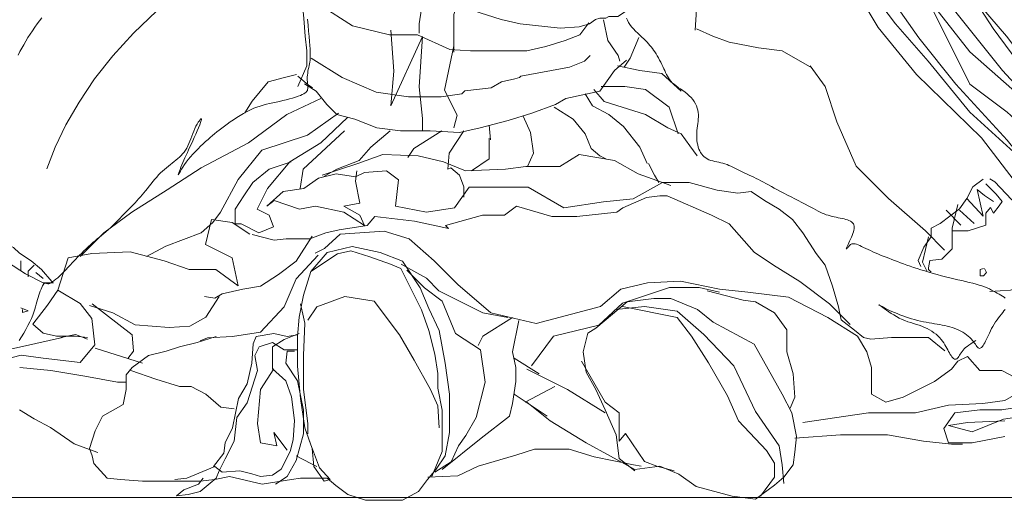
# Model space of a CAD drawing. Units: inches. Extents: x -17 to 1735, y -531 to 60.
# Tile 20 of 27: x 1734.798847 to 1734.807124, y -150.214646 to -150.210609. Entities that reach past the tile are written whole.
import ezdxf

# ---------------------------------------------------------------- set-up
doc = ezdxf.new("R2010")
doc.units = ezdxf.units.IN
doc.header["$MEASUREMENT"] = 0
doc.layers.add('A-FURN', color=242, linetype='Continuous', lineweight=18, true_color=0xcd2027)

# ---------------------------------------------------------------- blocks, each defined once
blk = doc.blocks.new('childrens_room_2')
blk.add_line((73.63163, 54.20212), (73.14631, 54.20212))
for points in [[(73.31539, 54.3045), (73.3149, 54.30385), (73.3144, 54.30318), (73.3139, 54.30247), (73.31339, 54.30174), (73.3129, 54.301), (73.31242, 54.30026), (73.31195, 54.29951), (73.31151, 54.29876), (73.31109, 54.29802), (73.31069, 54.29728), (73.31032, 54.29655)], [(73.31055, 54.23567), (73.31104, 54.23641), (73.31152, 54.23719), (73.31198, 54.238), (73.31242, 54.23882), (73.31281, 54.23962), (73.31315, 54.24037), (73.31344, 54.24107), (73.31368, 54.24171), (73.31387, 54.2423), (73.31404, 54.24286), (73.31418, 54.24338), (73.31431, 54.24388), (73.31444, 54.24436), (73.31457, 54.24483), (73.31471, 54.2453), (73.31487, 54.24576), (73.31503, 54.2462), (73.3152, 54.24661), (73.31537, 54.24698), (73.31553, 54.24729), (73.31569, 54.24754), (73.31583, 54.24772), (73.31596, 54.24782), (73.31609, 54.24785), (73.31621, 54.24785), (73.31634, 54.24781), (73.31649, 54.24777), (73.31666, 54.24775), (73.31686, 54.24776), (73.31709, 54.24782), (73.31737, 54.24796), (73.31768, 54.24816), (73.31802, 54.24841), (73.31839, 54.2487), (73.31876, 54.24902), (73.31914, 54.24937), (73.31951, 54.24972), (73.31988, 54.25008), (73.32022, 54.25043), (73.32056, 54.25078), (73.32088, 54.25112), (73.3212, 54.25147), (73.32153, 54.25182), (73.32187, 54.25219), (73.32223, 54.25257), (73.32261, 54.25297), (73.32302, 54.25339), (73.32345, 54.25384), (73.3239, 54.25429), (73.32437, 54.25475), (73.32485, 54.25521), (73.32533, 54.25567), (73.32581, 54.25611), (73.32629, 54.25654), (73.32676, 54.25694), (73.32722, 54.25732), (73.32768, 54.2577), (73.32813, 54.25807), (73.32859, 54.25845), (73.32906, 54.25884), (73.32953, 54.25925), (73.33002, 54.25969), (73.33052, 54.26015), (73.33103, 54.26065), (73.33154, 54.26116), (73.33206, 54.26169), (73.33256, 54.26221), (73.33306, 54.26273), (73.33355, 54.26324), (73.33401, 54.26373), (73.33445, 54.26419), (73.33488, 54.26462), (73.33528, 54.26504), (73.33567, 54.26545), (73.33605, 54.26586), (73.33642, 54.26627), (73.33679, 54.2667), (73.33717, 54.26714), (73.33754, 54.2676), (73.33792, 54.26808), (73.33831, 54.26858), (73.3387, 54.26907), (73.3391, 54.26957), (73.3395, 54.27005), (73.33991, 54.27052), (73.34032, 54.27097), (73.34074, 54.27139), (73.34115, 54.27178), (73.34157, 54.27215), (73.34199, 54.27251), (73.34241, 54.27284), (73.34282, 54.27317), (73.34323, 54.27349), (73.34363, 54.2738), (73.34402, 54.27412), (73.3444, 54.27444), (73.34476, 54.27477), (73.34511, 54.27511), (73.34544, 54.27547), (73.34575, 54.27585), (73.34604, 54.27625), (73.34631, 54.27669), (73.34655, 54.27716), (73.34678, 54.27766), (73.34699, 54.27817), (73.3472, 54.2787), (73.3474, 54.27924), (73.3476, 54.27978), (73.34782, 54.28032), (73.34804, 54.28084), (73.34829, 54.28134), (73.34854, 54.2818), (73.34878, 54.28221), (73.34901, 54.28254), (73.3492, 54.28279), (73.34935, 54.28293), (73.34944, 54.28295), (73.34946, 54.28283), (73.3494, 54.28256), (73.34927, 54.28215), (73.34908, 54.28164), (73.34884, 54.28104), (73.34856, 54.28038), (73.34826, 54.27968), (73.34794, 54.27897), (73.34762, 54.27827), (73.34731, 54.27759), (73.34701, 54.27695), (73.34672, 54.27634), (73.34645, 54.27575), (73.34618, 54.27519), (73.34593, 54.27464), (73.34569, 54.27411), (73.34547, 54.27359), (73.34526, 54.27309), (73.34507, 54.27261), (73.3449, 54.27216), (73.34476, 54.27177), (73.34465, 54.27144), (73.34457, 54.27119), (73.34452, 54.27103), (73.34452, 54.27097), (73.34457, 54.27103), (73.34465, 54.27119), (73.34479, 54.27145), (73.34497, 54.27178), (73.3452, 54.27219), (73.34548, 54.27265), (73.34582, 54.27316), (73.3462, 54.2737), (73.34664, 54.27426), (73.34713, 54.27483), (73.34764, 54.27541), (73.34818, 54.27598), (73.34873, 54.27655), (73.34929, 54.27709), (73.34983, 54.27762), (73.35036, 54.27811), (73.35086, 54.27856), (73.35133, 54.27899), (73.3518, 54.27939), (73.35227, 54.27977), (73.35275, 54.28016), (73.35325, 54.28054), (73.35378, 54.28094), (73.35435, 54.28136), (73.35496, 54.28181), (73.35562, 54.28227), (73.35631, 54.28275), (73.35702, 54.28322), (73.35774, 54.28368), (73.35847, 54.28411), (73.3592, 54.28452), (73.35992, 54.28488), (73.36062, 54.28519), (73.36131, 54.28545), (73.36198, 54.28567), (73.36265, 54.28587), (73.36332, 54.28604), (73.364, 54.2862), (73.36468, 54.28635), (73.36539, 54.28651), (73.3661, 54.28667), (73.36683, 54.28684), (73.36754, 54.28701), (73.36824, 54.28719), (73.36891, 54.28738), (73.36953, 54.28756), (73.37009, 54.28774), (73.37059, 54.28792), (73.371, 54.2881), (73.37134, 54.28827), (73.3716, 54.28845), (73.37181, 54.28862), (73.37196, 54.28881), (73.37207, 54.28901), (73.37213, 54.28922), (73.37216, 54.28944), (73.37217, 54.28969), (73.37216, 54.28996), (73.37214, 54.29024), (73.37211, 54.29054), (73.37208, 54.29086), (73.37206, 54.29119), (73.37205, 54.29154), (73.37206, 54.29191), (73.37209, 54.29229), (73.37214, 54.29268), (73.37221, 54.29308), (73.37228, 54.29349), (73.37236, 54.29389), (73.37244, 54.29429), (73.37252, 54.29468), (73.37258, 54.29506), (73.37264, 54.29543), (73.37267, 54.29581), (73.37269, 54.29622), (73.3727, 54.29667), (73.37268, 54.29721), (73.37265, 54.29784), (73.3726, 54.29858), (73.37253, 54.29947), (73.37244, 54.30051), (73.37234, 54.30167), (73.37222, 54.30291), (73.37208, 54.30419)], [(73.45448, 54.41111), (73.45858, 54.40576), (73.46299, 54.39757), (73.46709, 54.3897), (73.47119, 54.38214), (73.47718, 54.3708), (73.48475, 54.36198), (73.49042, 54.35222), (73.49894, 54.33301), (73.50907, 54.3176), (73.5138, 54.30941), (73.52137, 54.3006), (73.52894, 54.29052), (73.53745, 54.28044), (73.54596, 54.26974), (73.55353, 54.26029), (73.56456, 54.24769), (73.56734, 54.24595)], [(73.44696, 54.40942), (73.45988, 54.3985), (73.46883, 54.37369), (73.47578, 54.36277), (73.48473, 54.34887), (73.49268, 54.33497), (73.50163, 54.32108), (73.50858, 54.30817), (73.52051, 54.29328), (73.53144, 54.28137), (73.54138, 54.27244), (73.54734, 54.26052), (73.56316, 54.2436)], [(73.42106, 54.40855), (73.42295, 54.40603), (73.42737, 54.39974), (73.43241, 54.39344), (73.44093, 54.38273), (73.44629, 54.37958), (73.45259, 54.37423), (73.45701, 54.36919), (73.46079, 54.36226), (73.46489, 54.35502), (73.46741, 54.34746), (73.46962, 54.34116), (73.47183, 54.33487), (73.47592, 54.32731), (73.48002, 54.32196), (73.48009, 54.32041), (73.48639, 54.31506), (73.49396, 54.30246), (73.50216, 54.29239), (73.51603, 54.27885), (73.52738, 54.26405), (73.54189, 54.24704), (73.54565, 54.24155)], [(73.42509, 54.40843), (73.43702, 54.39652), (73.44994, 54.38163), (73.46088, 54.36376), (73.46783, 54.34887), (73.47479, 54.34291), (73.48175, 54.32505), (73.4887, 54.31512), (73.49765, 54.30321), (73.50461, 54.29527), (73.51355, 54.28435), (73.52448, 54.27442), (73.53343, 54.26549), (73.54138, 54.25358), (73.55157, 54.24155)], [(73.441, 54.40843), (73.44795, 54.40148), (73.45392, 54.38758), (73.46286, 54.37369), (73.46883, 54.35979), (73.47678, 54.34688), (73.48572, 54.33497), (73.49367, 54.32008), (73.5056, 54.30619), (73.51355, 54.2903), (73.5215, 54.28435), (73.53244, 54.27442), (73.53343, 54.27045), (73.54834, 54.25655), (73.55927, 54.24266), (73.5601, 54.24155)], [(73.45094, 54.40843), (73.45789, 54.40049), (73.46584, 54.38858), (73.4738, 54.36277), (73.46982, 54.37766), (73.47877, 54.36475), (73.48572, 54.35086), (73.49268, 54.34192), (73.50063, 54.32703), (73.50958, 54.31611), (73.51852, 54.30222), (73.53244, 54.28336), (73.54436, 54.26946), (73.55629, 54.25556), (73.56679, 54.24595)], [(73.43802, 54.40644), (73.44895, 54.39354), (73.46783, 54.35582), (73.4738, 54.34788), (73.48175, 54.332), (73.4897, 54.32008), (73.49566, 54.31016), (73.50262, 54.30023), (73.51057, 54.2903), (73.5215, 54.27839), (73.52945, 54.26847), (73.53741, 54.26052), (73.54238, 54.25655), (73.54933, 54.24663), (73.55079, 54.24155)], [(73.47578, 54.35185), (73.48672, 54.33696), (73.49765, 54.32306), (73.50262, 54.31115), (73.51355, 54.29725), (73.5225, 54.28931), (73.53343, 54.27541), (73.5384, 54.26847), (73.54436, 54.26449), (73.54834, 54.26052)], [(73.40269, 54.3308), (73.39865, 54.32205), (73.3973, 54.31196), (73.39596, 54.30321), (73.39596, 54.30119), (73.39596, 54.30119)], [(73.40943, 54.32743), (73.40876, 54.32138), (73.40606, 54.3133), (73.40337, 54.30523), (73.40337, 54.30052), (73.40337, 54.29917), (73.40337, 54.29716)], [(73.36676, 54.32146), (73.37149, 54.31862), (73.37591, 54.31673), (73.37938, 54.31642), (73.3819, 54.31516), (73.38568, 54.31296), (73.38915, 54.31233), (73.39419, 54.31044), (73.39829, 54.30981), (73.40302, 54.30729), (73.40744, 54.30603), (73.41343, 54.30414), (73.41753, 54.30319), (73.42604, 54.30225), (73.43014, 54.30256), (73.43235, 54.30319), (73.43361, 54.30414), (73.43455, 54.30445), (73.4355, 54.30445), (73.43581, 54.30445), (73.43644, 54.30477), (73.43834, 54.30477), (73.43999, 54.30587)], [(73.45329, 54.3223), (73.4536, 54.31884), (73.45581, 54.31475), (73.45644, 54.31065), (73.45518, 54.30624), (73.45486, 54.30183)], [(73.3691, 54.31443), (73.37005, 54.31097), (73.37099, 54.30813), (73.37131, 54.30435), (73.37162, 54.30057), (73.37194, 54.29743), (73.37194, 54.29428), (73.37005, 54.28987)], [(73.34543, 54.31061), (73.3399, 54.30598), (73.33493, 54.30121), (73.33052, 54.29635), (73.32665, 54.29144), (73.32332, 54.28652), (73.32051, 54.28166), (73.31823, 54.27689), (73.31646, 54.27226)], [(73.37131, 54.31128), (73.37478, 54.30719), (73.38171, 54.30278), (73.3896, 54.30089), (73.39559, 54.30089), (73.40252, 54.29774), (73.40694, 54.29743), (73.41261, 54.29743), (73.41892, 54.29743), (73.42302, 54.29837), (73.42712, 54.29963), (73.43027, 54.30089), (73.43216, 54.30341)], [(73.44023, 54.30444), (73.44041, 54.30398), (73.44065, 54.30351), (73.44096, 54.30304), (73.44132, 54.30257), (73.44173, 54.30211), (73.44216, 54.30165), (73.44261, 54.30121), (73.44306, 54.30078), (73.44349, 54.30038), (73.44391, 54.29999), (73.44428, 54.29963), (73.44462, 54.29928), (73.44494, 54.29895), (73.44523, 54.29862), (73.4455, 54.29829), (73.44576, 54.29795), (73.44602, 54.29759), (73.44627, 54.29721), (73.44653, 54.2968), (73.44679, 54.29637), (73.44705, 54.29592), (73.4473, 54.29547), (73.44755, 54.295), (73.44779, 54.29454), (73.44801, 54.29408), (73.44822, 54.29364), (73.4484, 54.29322), (73.44858, 54.29281), (73.44876, 54.29242), (73.44895, 54.29205), (73.44916, 54.29168), (73.4494, 54.29133), (73.44968, 54.29099), (73.45, 54.29065), (73.45038, 54.29032), (73.45081, 54.28999), (73.45127, 54.28965), (73.45176, 54.28932), (73.45225, 54.28897), (73.45273, 54.28862), (73.45319, 54.28825), (73.45363, 54.28787), (73.45402, 54.28747), (73.45437, 54.28704), (73.45467, 54.28661), (73.45493, 54.28616), (73.45514, 54.28571), (73.45531, 54.28524), (73.45544, 54.28477), (73.45552, 54.2843), (73.45556, 54.28383), (73.45556, 54.28335), (73.45553, 54.28288), (73.45549, 54.2824), (73.45543, 54.28191), (73.45536, 54.28142), (73.4553, 54.28092), (73.45526, 54.28042), (73.45523, 54.2799), (73.45522, 54.27938), (73.45523, 54.27886), (73.45527, 54.27835), (73.45533, 54.27785), (73.45542, 54.27737), (73.45553, 54.27691), (73.45568, 54.27648), (73.45585, 54.27608), (73.45605, 54.27572), (73.45628, 54.27539), (73.45654, 54.27509), (73.45682, 54.27483), (73.45713, 54.2746), (73.45747, 54.27439), (73.45783, 54.27422), (73.45822, 54.27408), (73.45862, 54.27396), (73.45905, 54.27385), (73.45948, 54.27376), (73.45992, 54.27366), (73.46037, 54.27357), (73.46081, 54.27346), (73.46125, 54.27333), (73.46168, 54.27318), (73.4621, 54.27301), (73.46252, 54.27282), (73.46293, 54.27262), (73.46334, 54.27241), (73.46376, 54.27219), (73.46418, 54.27197), (73.46461, 54.27176), (73.46505, 54.27154), (73.4655, 54.27133), (73.46596, 54.27112), (73.46642, 54.2709), (73.4669, 54.27068), (73.46739, 54.27046), (73.46789, 54.27022), (73.46839, 54.26997), (73.46891, 54.26971), (73.46944, 54.26943), (73.46999, 54.26914), (73.47056, 54.26883), (73.47116, 54.26851), (73.47178, 54.26817), (73.47243, 54.26782), (73.47312, 54.26745), (73.47385, 54.26707), (73.47461, 54.26668), (73.47537, 54.26629), (73.47615, 54.26589), (73.47691, 54.2655), (73.47765, 54.26512), (73.47835, 54.26475), (73.47901, 54.26441), (73.47961, 54.26409), (73.48016, 54.26379), (73.48067, 54.26351), (73.48115, 54.26326), (73.4816, 54.26304), (73.48203, 54.26283), (73.48245, 54.26265), (73.48287, 54.26249), (73.48329, 54.26235), (73.48373, 54.26223), (73.48416, 54.26212), (73.48459, 54.26203), (73.48502, 54.26194), (73.48545, 54.26185), (73.48587, 54.26177), (73.48627, 54.26168), (73.48667, 54.26159), (73.48705, 54.26149), (73.4874, 54.26137), (73.48773, 54.26124), (73.48803, 54.2611), (73.48828, 54.26094), (73.4885, 54.26075), (73.48866, 54.26055), (73.48877, 54.26032), (73.48884, 54.26007), (73.48885, 54.25979), (73.48883, 54.25949), (73.48876, 54.25917), (73.48867, 54.25883), (73.48855, 54.25847), (73.4884, 54.25808), (73.48823, 54.25768), (73.48806, 54.25727), (73.48787, 54.25687), (73.4877, 54.25648), (73.48753, 54.25613), (73.48739, 54.25581), (73.48727, 54.25555), (73.48719, 54.25535), (73.48715, 54.25523), (73.48715, 54.25518), (73.48719, 54.25519), (73.48725, 54.25524), (73.48733, 54.25533), (73.48743, 54.25545), (73.48755, 54.25558), (73.48766, 54.25572), (73.48778, 54.25586), (73.48791, 54.25598), (73.48804, 54.25609), (73.48819, 54.25618), (73.48836, 54.25625), (73.48855, 54.25628), (73.48877, 54.25628), (73.48903, 54.25625), (73.48932, 54.25617), (73.48966, 54.25605), (73.49002, 54.2559), (73.49042, 54.25572), (73.49085, 54.25551), (73.49131, 54.25529), (73.49179, 54.25506), (73.49229, 54.25483), (73.49281, 54.25459), (73.49335, 54.25436), (73.49391, 54.25412), (73.49448, 54.25388), (73.49506, 54.25365), (73.49565, 54.25341), (73.49625, 54.25318), (73.49686, 54.25294), (73.49747, 54.2527), (73.4981, 54.25247), (73.49873, 54.25223), (73.49939, 54.25199), (73.50007, 54.25175), (73.50077, 54.2515), (73.5015, 54.25125), (73.50227, 54.251), (73.50308, 54.25074), (73.50392, 54.25048), (73.50478, 54.25022), (73.50567, 54.24996), (73.50657, 54.24971), (73.50747, 54.24946), (73.50837, 54.24923), (73.50926, 54.249), (73.51014, 54.24879), (73.511, 54.2486), (73.51184, 54.24841), (73.51264, 54.24822), (73.51342, 54.24804), (73.51416, 54.24786), (73.51486, 54.24767), (73.51551, 54.24748), (73.51612, 54.24728), (73.51668, 54.24707), (73.51721, 54.24686), (73.5177, 54.24664), (73.51815, 54.24641), (73.51859, 54.24619), (73.519, 54.24597), (73.5194, 54.24575), (73.51979, 54.24554), (73.52016, 54.24533), (73.52051, 54.24512), (73.52083, 54.24491), (73.52111, 54.2447)], [(73.52107, 54.24229), (73.52082, 54.24197), (73.52055, 54.24162), (73.52027, 54.24126), (73.51997, 54.24086), (73.51966, 54.24046), (73.51935, 54.24003), (73.51904, 54.23959), (73.51874, 54.23913), (73.51846, 54.23866), (73.51819, 54.23819), (73.51794, 54.23771), (73.51771, 54.23723), (73.51749, 54.23677), (73.51729, 54.23632), (73.51709, 54.2359), (73.5169, 54.2355), (73.51672, 54.23515), (73.51655, 54.23484), (73.51638, 54.23457), (73.51621, 54.23435), (73.51605, 54.23418), (73.5159, 54.23405), (73.51575, 54.23398), (73.5156, 54.23396), (73.51546, 54.23399), (73.51533, 54.23408), (73.51519, 54.23421), (73.51505, 54.23439), (73.5149, 54.2346), (73.51473, 54.23484), (73.51455, 54.2351), (73.51434, 54.23538), (73.5141, 54.23567), (73.51382, 54.23597), (73.51352, 54.23627), (73.51318, 54.23656), (73.51282, 54.23685), (73.51244, 54.23713), (73.51203, 54.2374), (73.5116, 54.23765), (73.51115, 54.23788), (73.51069, 54.23808), (73.51022, 54.23826), (73.50973, 54.23843), (73.50923, 54.23857), (73.50872, 54.2387), (73.50819, 54.23882), (73.50765, 54.23893), (73.50711, 54.23903), (73.50655, 54.23913), (73.50598, 54.23922), (73.50541, 54.23932), (73.50482, 54.23942), (73.50422, 54.23953), (73.50362, 54.23964), (73.503, 54.23978), (73.50238, 54.23992), (73.50174, 54.24009), (73.5011, 54.24028), (73.50046, 54.24047), (73.49983, 54.24069), (73.4992, 54.24091), (73.49859, 54.24113), (73.498, 54.24137), (73.49744, 54.2416), (73.4969, 54.24184), (73.4964, 54.24207), (73.49593, 54.24229), (73.49551, 54.2425), (73.49514, 54.24269), (73.49481, 54.24287), (73.49455, 54.24301), (73.49434, 54.24313), (73.49419, 54.24321), (73.49411, 54.24325), (73.49409, 54.24326), (73.49414, 54.24322), (73.49425, 54.24315), (73.49443, 54.24303), (73.49466, 54.24287), (73.49497, 54.24265), (73.49533, 54.24239), (73.49576, 54.2421), (73.49623, 54.24177), (73.49674, 54.24143), (73.49729, 54.24109), (73.49786, 54.24075), (73.49846, 54.24043), (73.49907, 54.24013), (73.49968, 54.23988), (73.50029, 54.23965), (73.50091, 54.23945), (73.50152, 54.23926), (73.50212, 54.23907), (73.50271, 54.23888), (73.50329, 54.23868), (73.50385, 54.23845), (73.50439, 54.2382), (73.50491, 54.23793), (73.5054, 54.23763), (73.50587, 54.23731), (73.50631, 54.23697), (73.50672, 54.23662), (73.50709, 54.23625), (73.50742, 54.23588), (73.50772, 54.23551), (73.50798, 54.23513), (73.50822, 54.23475), (73.50843, 54.23438), (73.50862, 54.23402), (73.5088, 54.23366), (73.50898, 54.23332), (73.50916, 54.233), (73.50934, 54.23269), (73.50952, 54.23241), (73.5097, 54.23217), (73.50989, 54.23196), (73.51007, 54.2318), (73.51024, 54.23168), (73.51041, 54.23163), (73.51058, 54.23163), (73.51073, 54.2317), (73.51088, 54.23184), (73.51102, 54.23202), (73.51117, 54.23224), (73.51132, 54.23248), (73.51149, 54.23275), (73.51167, 54.23303), (73.51186, 54.23331), (73.51208, 54.23358), (73.51233, 54.23385), (73.51261, 54.23412), (73.51294, 54.23439), (73.51331, 54.23467), (73.51374, 54.23496), (73.51422, 54.23528), (73.51478, 54.23562)], [(73.43532, 54.30404), (73.43626, 54.29963), (73.43847, 54.29648), (73.43878, 54.29522)], [(73.38989, 54.30187), (73.39057, 54.29312), (73.38989, 54.28572)], [(73.45518, 54.30215), (73.45865, 54.30057), (73.46212, 54.29932), (73.46842, 54.29806), (73.47347, 54.29743), (73.47978, 54.29382)], [(73.38989, 54.28572), (73.39663, 54.30052), (73.39596, 54.28975), (73.39663, 54.28303), (73.39663, 54.28033)], [(73.44288, 54.30026), (73.44099, 54.29585), (73.43973, 54.29396)], [(73.40337, 54.2985), (73.40135, 54.28908), (73.40404, 54.2837), (73.40337, 54.28101)], [(73.4402, 54.29548), (73.43768, 54.29327), (73.43453, 54.28886), (73.42728, 54.28729), (73.42507, 54.28603), (73.42002, 54.28414), (73.41498, 54.28257), (73.40899, 54.28099), (73.40457, 54.28005), (73.39827, 54.28036), (73.39196, 54.28036), (73.38692, 54.28099), (73.38219, 54.28288), (73.3784, 54.28383), (73.3762, 54.28603), (73.37399, 54.28886), (73.37147, 54.29044)], [(73.37289, 54.29585), (73.37951, 54.29176), (73.38676, 54.28861), (73.3937, 54.28766), (73.40063, 54.28766), (73.40505, 54.28829), (73.40568, 54.28892), (73.41135, 54.28955), (73.41356, 54.29081), (73.4164, 54.29144), (73.41734, 54.29176), (73.41766, 54.29207), (73.42806, 54.29396), (73.43122, 54.29522), (73.43248, 54.29648)], [(73.43831, 54.29422), (73.44304, 54.29327), (73.44777, 54.29264), (73.45187, 54.28886)], [(73.47946, 54.29428), (73.48261, 54.28987), (73.48513, 54.28231), (73.48923, 54.27286), (73.49617, 54.26594), (73.50405, 54.25901), (73.50815, 54.25491)], [(73.36973, 54.29239), (73.36721, 54.29176), (73.36374, 54.29081), (73.36027, 54.28672), (73.3587, 54.2842)], [(73.37005, 54.29207), (73.37226, 54.29018), (73.3732, 54.28955)], [(73.43327, 54.28918), (73.43547, 54.28666), (73.43926, 54.2854), (73.4443, 54.28383), (73.44903, 54.28099), (73.45187, 54.27973), (73.45376, 54.27721), (73.45534, 54.27501)], [(73.43484, 54.28981), (73.43989, 54.28981), (73.4443, 54.28918), (73.44935, 54.2854), (73.45124, 54.27973)], [(73.37494, 54.28729), (73.36768, 54.28383), (73.35949, 54.27784), (73.3494, 54.27249), (73.34215, 54.26777), (73.33458, 54.26304), (73.32859, 54.25863), (73.32354, 54.2536)], [(73.43137, 54.28824), (73.43295, 54.28572), (73.43642, 54.28383), (73.43957, 54.28131), (73.44304, 54.2769), (73.44462, 54.27343)], [(73.42475, 54.2854), (73.42885, 54.28288), (73.43137, 54.27973), (73.43264, 54.27658), (73.43453, 54.27501), (73.43579, 54.27438)], [(73.37872, 54.28414), (73.3721, 54.27942), (73.36232, 54.27627), (73.35728, 54.26997), (73.3535, 54.26304), (73.35192, 54.26084), (73.3494, 54.25863), (73.34183, 54.2558), (73.33773, 54.2536)], [(73.38061, 54.2832), (73.37494, 54.27784), (73.36832, 54.27375), (73.36359, 54.26808), (73.36138, 54.26367), (73.3639, 54.26241), (73.36485, 54.25989), (73.36169, 54.25863), (73.35791, 54.26052), (73.35665, 54.26052), (73.35665, 54.26052), (73.35665, 54.26367), (73.35854, 54.26651), (73.36043, 54.26934), (73.3639, 54.27218), (73.36863, 54.27375)], [(73.41813, 54.28351), (73.41971, 54.28005), (73.42034, 54.27564), (73.41908, 54.2728)], [(73.41088, 54.28162), (73.4112, 54.27847)], [(73.37998, 54.28036), (73.37115, 54.27218), (73.37052, 54.26808)], [(73.38976, 54.28036), (73.38566, 54.2769), (73.38313, 54.27406), (73.3784, 54.27218), (73.37557, 54.2706)], [(73.40079, 54.28036), (73.3948, 54.27658), (73.39354, 54.27469)], [(73.40552, 54.28036), (73.40237, 54.27564), (73.40205, 54.27218), (73.40268, 54.27249), (73.40457, 54.27092), (73.40552, 54.2684), (73.40552, 54.26619)], [(73.41088, 54.27879), (73.41088, 54.27438), (73.4071, 54.27186)], [(73.37525, 54.27092), (73.38282, 54.27343), (73.38818, 54.27532), (73.39575, 54.27501), (73.40111, 54.27375), (73.40584, 54.27186), (73.41435, 54.27218), (73.41876, 54.2728), (73.42601, 54.2728), (73.43011, 54.27532), (73.43768, 54.27406), (73.44273, 54.27123), (73.44966, 54.26871)], [(73.44493, 54.27343), (73.44619, 54.27092), (73.44714, 54.26934)], [(73.50816, 54.23342), (73.50469, 54.23625), (73.50059, 54.23625), (73.49681, 54.23625), (73.49239, 54.23594), (73.49082, 54.23625), (73.48892, 54.23782), (73.48609, 54.24003), (73.48546, 54.24286), (73.4842, 54.24727), (73.48262, 54.25168), (73.48073, 54.2542), (73.47789, 54.25861), (73.47568, 54.26144), (73.47284, 54.26365), (73.46969, 54.26554), (73.46685, 54.26743), (73.46402, 54.26711), (73.4596, 54.26774), (73.45361, 54.26932), (73.44794, 54.26932), (73.44163, 54.26585), (73.43532, 54.26522), (73.42681, 54.26396), (73.41924, 54.26837), (73.40663, 54.26837), (73.40348, 54.26396), (73.39749, 54.26302), (73.39087, 54.26428), (73.3915, 54.26994), (73.38898, 54.27183), (73.38425, 54.27152), (73.38235, 54.27057), (73.37826, 54.2712), (73.37447, 54.27026), (73.37132, 54.26806), (73.3669, 54.26743), (73.36344, 54.26428), (73.36501, 54.26554), (73.37037, 54.26365), (73.37384, 54.26428), (73.37983, 54.26302), (73.38425, 54.26018), (73.3833, 54.26239), (73.37983, 54.26428), (73.3833, 54.26491), (73.38235, 54.26963), (73.38267, 54.27183)], [(73.51778, 54.27017), (73.51889, 54.26951), (73.52246, 54.26572), (73.52669, 54.26238), (73.53003, 54.26038), (73.53293, 54.25882), (73.53471, 54.25904), (73.53404, 54.25704), (73.53248, 54.25437), (73.53137, 54.25326), (73.53271, 54.25214), (73.53226, 54.25125), (73.52981, 54.25125), (73.5278, 54.24947), (73.52602, 54.24769), (73.52223, 54.24636), (73.51778, 54.24613)], [(73.51635, 54.27003), (73.51414, 54.26845), (73.51288, 54.26594), (73.5113, 54.26373), (73.5072, 54.26058), (73.50531, 54.25964), (73.50531, 54.25775), (73.50373, 54.25554), (73.50247, 54.25271), (73.5031, 54.25145)], [(73.51698, 54.26908), (73.51918, 54.26688), (73.52045, 54.26531), (73.51982, 54.26436), (73.51855, 54.26279), (73.51792, 54.26405), (73.51698, 54.26279), (73.51698, 54.26153), (73.51698, 54.26027), (73.51319, 54.25901), (73.5113, 54.25901), (73.50973, 54.25901), (73.50973, 54.25712), (73.50973, 54.25523), (73.50752, 54.25302), (73.505, 54.25271), (73.50468, 54.25114), (73.50468, 54.25082), (73.50531, 54.25019)], [(73.30021, 54.26473), (73.3002, 54.26369), (73.29957, 54.26716), (73.29641, 54.2659), (73.29641, 54.26558), (73.29862, 54.26243), (73.29736, 54.26306), (73.29988, 54.26054), (73.30303, 54.25519), (73.30619, 54.25425), (73.30808, 54.25236), (73.31186, 54.24984), (73.31565, 54.24795), (73.31785, 54.24795)], [(73.29894, 54.26684), (73.30083, 54.26369), (73.30209, 54.26243), (73.30303, 54.26117), (73.30524, 54.25803), (73.30682, 54.25677), (73.30934, 54.25551), (73.3106, 54.25425), (73.31312, 54.25267), (73.31533, 54.25078), (73.31754, 54.24826)], [(73.36028, 54.25829), (73.36501, 54.25703), (73.36753, 54.25735), (73.37258, 54.25735), (73.37605, 54.25861), (73.37889, 54.25924), (73.38488, 54.26018), (73.38645, 54.26207), (73.39497, 54.26113), (73.40222, 54.25955), (73.40159, 54.26018), (73.40947, 54.26239), (73.4142, 54.26239), (73.41672, 54.26428), (73.42429, 54.26207), (73.42965, 54.26207), (73.43816, 54.26302), (73.43942, 54.26396), (73.44447, 54.26617), (73.44731, 54.26648), (73.44888, 54.26648), (73.45834, 54.26239), (73.46212, 54.2605), (73.46748, 54.25451), (73.47158, 54.25168), (73.47726, 54.24822), (73.48356, 54.24349), (73.48798, 54.23908)], [(73.51635, 54.26216), (73.51509, 54.26783), (73.51666, 54.26657), (73.51855, 54.26531)], [(73.51099, 54.26468), (73.50973, 54.25964), (73.50973, 54.25869)], [(73.51288, 54.26594), (73.51635, 54.26216)], [(73.50846, 54.26342), (73.51162, 54.26027)], [(73.5113, 54.26342), (73.51446, 54.26058)], [(73.3598, 54.25832), (73.35602, 54.26084), (73.3516, 54.26147), (73.35034, 54.25612), (73.35602, 54.25328), (73.35728, 54.2473), (73.35255, 54.25076), (73.34687, 54.25076), (73.34151, 54.25265), (73.33426, 54.25454), (73.32607, 54.25423), (73.32102, 54.25328), (73.31881, 54.24635), (73.32354, 54.24352), (73.32607, 54.24037), (73.3267, 54.2347), (73.32354, 54.23092), (73.31566, 54.23187), (73.31093, 54.2325), (73.30715, 54.23155)], [(73.31062, 54.22085), (73.31377, 54.21896), (73.31724, 54.21707), (73.32228, 54.2136), (73.3248, 54.21266), (73.32733, 54.21171)], [(73.37313, 54.25792), (73.36966, 54.25256), (73.36588, 54.24973), (73.36209, 54.24721), (73.35831, 54.24658), (73.35389, 54.24563), (73.35232, 54.24469), (73.35011, 54.245)], [(73.37372, 54.25429), (73.37573, 54.25529), (73.37908, 54.2583), (73.38845, 54.25897), (73.39381, 54.2573), (73.39916, 54.25261), (73.40419, 54.2476), (73.41122, 54.24158), (73.42093, 54.23924), (73.43465, 54.24292), (73.439, 54.24659), (73.4447, 54.24793), (73.45173, 54.24827), (73.4601, 54.24659), (73.46612, 54.24593), (73.47483, 54.24492), (73.4832, 54.24058), (73.48956, 54.23656), (73.49157, 54.23322), (73.49257, 54.22988), (73.49257, 54.22419), (73.49559, 54.22252), (73.49927, 54.22352), (73.50597, 54.22687), (73.50965, 54.22954), (73.51099, 54.23121), (73.513, 54.23222), (73.51567, 54.22921), (73.52036, 54.22921), (73.52739, 54.22553)], [(73.52103, 54.21516), (73.514, 54.21383), (73.50898, 54.21383), (73.50797, 54.21684), (73.51032, 54.22018), (73.51567, 54.22085), (73.52036, 54.22085), (73.52438, 54.22152)], [(73.52103, 54.21851), (73.513, 54.21817), (73.50898, 54.2175), (73.514, 54.21617), (73.5207, 54.21884), (73.52304, 54.21918)], [(73.50468, 54.25775), (73.50342, 54.25239), (73.50437, 54.25051)], [(73.33466, 54.22989), (73.3334, 54.22832), (73.3334, 54.22517), (73.33277, 54.22202), (73.32836, 54.2195), (73.32678, 54.21635), (73.32552, 54.21257), (73.32615, 54.211), (73.32646, 54.20942), (73.3293, 54.20627), (73.33214, 54.20596), (73.33687, 54.20564), (73.3416, 54.20564), (73.34507, 54.20564), (73.34917, 54.20564), (73.35232, 54.20596), (73.35547, 54.20659), (73.36241, 54.20501), (73.36871, 54.20596), (73.37061, 54.20627), (73.37628, 54.20627), (73.37817, 54.2047), (73.38069, 54.20281), (73.38448, 54.20155), (73.38826, 54.20155), (73.39236, 54.20155), (73.39583, 54.20344), (73.39772, 54.20596), (73.39961, 54.20816), (73.4015, 54.211), (73.40245, 54.21603), (73.40245, 54.22422), (73.4015, 54.23083), (73.40024, 54.23776), (73.39804, 54.24249), (73.39614, 54.24689), (73.39236, 54.25256), (73.38763, 54.25445), (73.38164, 54.25571), (73.37628, 54.25445), (73.37281, 54.25036), (73.37124, 54.24532), (73.37029, 54.2406), (73.36997, 54.2365), (73.36997, 54.2302), (73.37061, 54.22328), (73.37155, 54.21698), (73.37313, 54.21257), (73.37344, 54.20879), (73.37565, 54.20564), (73.37691, 54.20596), (73.3747, 54.20848), (73.3725, 54.21414)], [(73.37439, 54.25382), (73.36966, 54.24878), (73.36714, 54.2428), (73.36209, 54.23745), (73.3561, 54.2365), (73.35074, 54.23619), (73.34917, 54.23556)], [(73.37281, 54.25036), (73.37849, 54.25414), (73.38133, 54.25477), (73.38542, 54.25351), (73.38984, 54.25193), (73.39205, 54.25099), (73.39488, 54.24532), (73.39646, 54.24217), (73.39804, 54.23776), (73.3993, 54.23272), (73.39993, 54.22863), (73.39993, 54.22548), (73.40087, 54.22076), (73.40087, 54.21603), (73.40087, 54.21194), (73.39867, 54.20659)], [(73.31092, 54.25267), (73.31092, 54.25047)], [(73.31375, 54.25173), (73.31249, 54.25047), (73.31249, 54.24921)], [(73.39213, 54.25194), (73.39749, 54.24894), (73.40017, 54.24626), (73.40954, 54.24158), (73.4149, 54.24058)], [(73.31407, 54.25015), (73.31565, 54.24889)], [(73.3993, 54.20753), (73.40277, 54.20974), (73.40434, 54.2132), (73.40592, 54.2154), (73.40813, 54.21918), (73.41002, 54.22674), (73.40907, 54.23367), (73.40371, 54.23713), (73.40087, 54.24406), (73.39709, 54.24689), (73.39331, 54.25067)], [(73.51644, 54.25103), (73.51577, 54.25081), (73.51577, 54.24947), (73.51644, 54.24947), (73.51711, 54.25014), (73.51666, 54.25103)], [(73.31881, 54.24635), (73.31661, 54.2432), (73.31345, 54.23911), (73.31566, 54.23722), (73.3185, 54.23659), (73.3226, 54.23659), (73.32512, 54.23628)], [(73.32552, 54.24312), (73.33056, 54.24154), (73.33529, 54.23902), (73.34254, 54.23839), (73.34696, 54.23871), (73.35043, 54.2406), (73.35326, 54.245)], [(73.37218, 54.23997), (73.37407, 54.2428), (73.38006, 54.245), (73.38637, 54.24406), (73.39173, 54.23682), (73.39488, 54.23146), (73.39835, 54.22517), (73.39993, 54.2217), (73.40024, 54.21698)], [(73.41992, 54.23021), (73.42461, 54.23656), (73.43432, 54.2389), (73.43934, 54.24359), (73.44938, 54.24693), (73.45574, 54.24693), (73.4601, 54.24593)], [(73.45742, 54.24626), (73.46512, 54.24425), (73.4678, 54.24392), (73.47182, 54.24158), (73.47449, 54.2379), (73.47449, 54.23322), (73.47583, 54.22854), (73.47617, 54.22352), (73.47516, 54.22118)], [(73.32615, 54.24343), (73.33466, 54.23682), (73.33498, 54.23335), (73.33372, 54.23178)], [(73.37061, 54.24343), (73.37124, 54.2406), (73.37155, 54.23934), (73.37124, 54.23241), (73.37124, 54.22517), (73.37218, 54.21792), (73.37218, 54.21572)], [(73.41892, 54.22252), (73.42394, 54.21851), (73.43164, 54.21383), (73.44202, 54.20814), (73.44737, 54.20881), (73.45139, 54.20714), (73.45508, 54.20446), (73.46278, 54.20246), (73.4678, 54.20179), (73.47182, 54.2048), (73.47382, 54.20647), (73.47583, 54.20914), (73.47617, 54.21182), (73.4765, 54.21516), (73.4755, 54.22018), (73.47349, 54.22419), (73.46746, 54.23489), (73.45876, 54.23957), (73.45541, 54.24225), (73.44972, 54.24459), (73.44604, 54.24459), (73.44034, 54.24392), (73.43365, 54.23824), (73.43197, 54.23723), (73.43097, 54.23322), (73.43164, 54.22887), (73.43365, 54.22519), (73.43566, 54.22085), (73.438, 54.2155), (73.43867, 54.21048), (73.44202, 54.20781)], [(73.438, 54.24225), (73.44403, 54.24292), (73.45106, 54.24191), (73.45675, 54.2369), (73.46311, 54.23021), (73.4678, 54.22051), (73.47282, 54.21316), (73.47349, 54.20914), (73.47382, 54.20513)], [(73.43934, 54.24292), (73.45106, 54.24058), (73.45407, 54.23656), (73.45775, 54.23088), (73.46177, 54.22386), (73.46411, 54.21851), (73.47014, 54.21215), (73.47182, 54.20948), (73.47182, 54.20647), (73.4688, 54.20246)], [(73.31123, 54.24228), (73.31123, 54.24165), (73.31249, 54.24197), (73.31092, 54.2426)], [(73.41724, 54.23991), (73.4159, 54.23322), (73.41657, 54.22988), (73.41657, 54.22687), (73.4159, 54.22219), (73.41523, 54.21951), (73.40921, 54.21483), (73.40084, 54.20814)], [(73.4159, 54.24058), (73.40954, 54.23656), (73.40854, 54.23456)], [(73.31944, 54.23628), (73.3226, 54.23691), (73.32512, 54.23596)], [(73.37029, 54.23713), (73.36714, 54.23587), (73.36461, 54.2343), (73.36461, 54.22957), (73.36745, 54.22706), (73.36871, 54.22359), (73.36934, 54.21855), (73.36903, 54.21446), (73.3684, 54.21194), (73.36651, 54.20816), (73.36461, 54.2069), (73.36209, 54.20659), (73.3602, 54.20722), (73.35768, 54.20785), (73.35389, 54.20753), (73.35232, 54.20879), (73.34633, 54.20627), (73.3438, 54.20596)], [(73.352, 54.20879), (73.35421, 54.21163), (73.35453, 54.21383), (73.3561, 54.21698), (73.35673, 54.22013), (73.35736, 54.22328), (73.35925, 54.22643), (73.3602, 54.23083), (73.36052, 54.23493), (73.36115, 54.2365), (73.36493, 54.23713), (73.36777, 54.2365), (73.36997, 54.23682)], [(73.31976, 54.23628), (73.31408, 54.23502), (73.30872, 54.23376), (73.3062, 54.23124), (73.3062, 54.22714)], [(73.33466, 54.22989), (73.33813, 54.23241), (73.34191, 54.23335), (73.34475, 54.2343), (73.34853, 54.23524), (73.35263, 54.2365)], [(73.36997, 54.23367), (73.36714, 54.23367), (73.36461, 54.23524), (73.36178, 54.2343), (73.36083, 54.23241), (73.36146, 54.22926), (73.35925, 54.22233), (73.35705, 54.21918), (73.35642, 54.21414), (73.35453, 54.21037), (73.35326, 54.20785), (73.35263, 54.20627), (73.34917, 54.20344), (73.34664, 54.20281), (73.34412, 54.20249), (73.3457, 54.20375), (73.34885, 54.20501), (73.3498, 54.20627)], [(73.32678, 54.23398), (73.33687, 54.23083)], [(73.36934, 54.23335), (73.36777, 54.23335), (73.36745, 54.23083), (73.36997, 54.22706), (73.37124, 54.22076), (73.37124, 54.21572), (73.36966, 54.21005), (73.36777, 54.20659), (73.36525, 54.20501)], [(73.41624, 54.23188), (73.42159, 54.22854)], [(73.43063, 54.23121), (73.43566, 54.22252), (73.43867, 54.22018), (73.43867, 54.21416), (73.44001, 54.21583), (73.44403, 54.20981), (73.44671, 54.20881), (73.45039, 54.20781)], [(73.3107, 54.22989), (73.31732, 54.22926), (73.32457, 54.228), (73.33151, 54.22674), (73.3334, 54.22674)], [(73.33435, 54.22926), (73.33971, 54.22737), (73.34475, 54.2258), (73.34727, 54.2258), (73.35043, 54.22422), (73.35358, 54.22139), (73.35642, 54.22107)], [(73.36493, 54.22957), (73.36209, 54.22517), (73.36146, 54.21792), (73.36209, 54.21383), (73.36556, 54.2132), (73.36493, 54.21603), (73.36777, 54.21226)], [(73.41892, 54.22954), (73.42762, 54.22519), (73.43566, 54.22018)], [(73.41624, 54.22419), (73.42327, 54.21951)], [(73.41858, 54.22252), (73.42494, 54.22586)], [(73.47784, 54.21817), (73.4919, 54.22018), (73.50195, 54.22018), (73.50898, 54.22185), (73.51634, 54.22219), (73.52103, 54.22285), (73.52337, 54.22419), (73.52773, 54.22419), (73.53074, 54.22419)], [(73.47617, 54.21483), (73.48588, 54.2155), (73.49592, 54.2155), (73.50362, 54.21416), (73.50965, 54.21349), (73.51199, 54.21349)], [(73.39782, 54.20647), (73.40419, 54.2068), (73.40854, 54.20881), (73.41657, 54.21115), (73.42059, 54.21249), (73.42796, 54.21249), (73.43331, 54.21082), (73.44168, 54.20914), (73.44336, 54.20881)], [(73.36966, 54.211), (73.37281, 54.20942), (73.37407, 54.20879)]]:
    blk.add_lwpolyline(points)

msp = doc.modelspace()

# ---------------------------------------------------------------- block references
at = {"layer": 'A-FURN', "xscale": 0.0393700787401575, "yscale": 0.0393700787401575, "zscale": 0.0393700787401575}
msp.add_blockref('childrens_room_2', (1731.9126009, -152.348565), dxfattribs=at)

doc.saveas('drawing.dxf')
